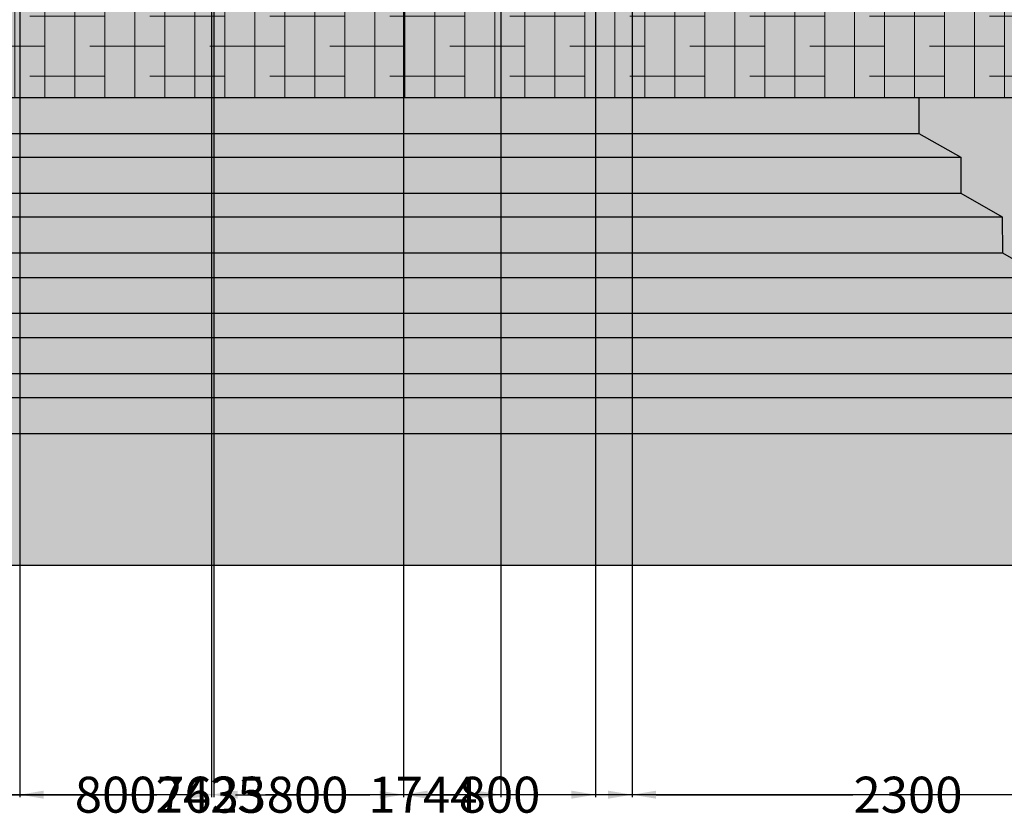
# Model space of a CAD drawing. Units: millimetres. Extents: x 11032 to 26788, y 3406 to 24505.
# Tile 12 of 78: x 17145 to 21249, y 3406 to 6736. Entities that reach past the tile are written whole.
import ezdxf

# ---------------------------------------------------------------- set-up
doc = ezdxf.new("R2010")
doc.units = ezdxf.units.MM
doc.header["$MEASUREMENT"] = 0
for name, color, linetype, lineweight in [('A-ANNO-DIMS', 2, 'Continuous', 18), ('A-FLOR-STRS', 7, 'Continuous', 25), ('A-FLOR-STRS-PATT', 8, 'Continuous', 13), ('A-WALL-PLIN', 7, 'Continuous', 30), ('A-WALL-PLIN-PATT', 253, 'Continuous', 13), ('L-PLNT-PATT', 92, 'Continuous', 13)]:
    doc.layers.add(name, color=color, linetype=linetype, lineweight=lineweight)
doc.styles.get("Standard").update_dxf_attribs({"font": 'arial.ttf'})
doc.dimstyles.get("Standard").update_dxf_attribs({"dimtxt": 150, "dimasz": 100, "dimexe": 10, "dimexo": 5, "dimgap": 5, "dimtad": 0, "dimtih": 1, "dimtoh": 1, "dimdec": 0, "dimzin": 0, "dimdsep": 46, "dimtxsty": 'Standard', "dimcen": 0.09, "dimadec": 0, "dimazin": 0, "dimtfac": 1, "dimtdec": 0, "dimtofl": 0, "dimtmove": 0, "dimatfit": 3, "dimfxl": 1, "dimtolj": 1, "dimtzin": 0, "dimarcsym": 0})

# ---------------------------------------------------------------- blocks, each defined once
blk = doc.blocks.new('*D36')
at = {"layer": 'A-ANNO-DIMS', "color": 0, "lineweight": -2, "transparency": 16777216}
for p, q in [((12301.3, 17115.9), (12301.3, 24416.9)), ((12401.3, 24406.9), (18569.2, 24406.9)), ((25297.4, 24406.9), (19129.5, 24406.9)), ((25397.4, 4466.4), (25397.4, 24416.9))]:
    blk.add_line(p, q, dxfattribs=at)
at = {"layer": 'A-ANNO-DIMS', "color": 0, "transparency": 16777216}
for points in [[(12401.3, 24423.5), (12401.3, 24390.2), (12301.3, 24406.9)], [(25297.4, 24423.5), (25297.4, 24390.2), (25397.4, 24406.9)]]:
    blk.add_solid(points, dxfattribs=at)
at = {"layer": 'Defpoints', "color": 0, "transparency": 16777216}
for p in [(25397.4, 24406.9), (12301.3, 17110.9), (25397.4, 4461.4)]:
    blk.add_point(p, dxfattribs=at)
at = {"layer": 'A-ANNO-DIMS', "color": 0, "transparency": 16777216, "insert": (18849.3, 24406.9), "char_height": 150, "attachment_point": 5}
blk.add_mtext('\\A1;13096', dxfattribs=at)
blk = doc.blocks.new('*D37')
at = {"layer": 'A-ANNO-DIMS', "color": 0, "lineweight": -2, "transparency": 16777216}
for p, q in [((18087.7, 23450.4), (11334.8, 23450.4)), ((11344.8, 23350.4), (11344.8, 14037.5)), ((11344.8, 4561.4), (11344.8, 13874.3)), ((12927.7, 4461.4), (11334.8, 4461.4))]:
    blk.add_line(p, q, dxfattribs=at)
at = {"layer": 'A-ANNO-DIMS', "color": 0, "transparency": 16777216}
for points in [[(11328.1, 23350.4), (11361.4, 23350.4), (11344.8, 23450.4)], [(11328.1, 4561.4), (11361.4, 4561.4), (11344.8, 4461.4)]]:
    blk.add_solid(points, dxfattribs=at)
at = {"layer": 'Defpoints', "color": 0, "transparency": 16777216}
for p in [(11344.8, 23450.4), (18092.7, 23450.4), (12932.7, 4461.4)]:
    blk.add_point(p, dxfattribs=at)
at = {"layer": 'A-ANNO-DIMS', "color": 0, "transparency": 16777216, "insert": (11344.8, 13955.9), "char_height": 150, "attachment_point": 5}
blk.add_mtext('\\A1;18989', dxfattribs=at)
blk = doc.blocks.new('*D49')
at = {"layer": 'A-ANNO-DIMS', "color": 0, "lineweight": -2, "transparency": 16777216}
for p, q in [((17953.5, 10206.4), (17953.5, 3494.9)), ((14996.4, 6406.4), (14996.4, 3494.9)), ((15096.4, 3504.9), (16244.7, 3504.9)), ((17853.5, 3504.9), (16705.2, 3504.9))]:
    blk.add_line(p, q, dxfattribs=at)
at = {"layer": 'A-ANNO-DIMS', "color": 0, "transparency": 16777216}
for points in [[(15096.4, 3521.6), (15096.4, 3488.2), (14996.4, 3504.9)], [(17853.5, 3521.6), (17853.5, 3488.2), (17953.5, 3504.9)]]:
    blk.add_solid(points, dxfattribs=at)
at = {"layer": 'Defpoints', "color": 0, "transparency": 16777216}
for p in [(17953.5, 10211.4), (14996.4, 6411.4), (17953.5, 3504.9)]:
    blk.add_point(p, dxfattribs=at)
at = {"layer": 'A-ANNO-DIMS', "color": 0, "transparency": 16777216, "insert": (16474.9, 3504.9), "char_height": 150, "attachment_point": 5}
blk.add_mtext('\\A1;2957', dxfattribs=at)
blk = doc.blocks.new('*D50')
at = {"layer": 'A-ANNO-DIMS', "color": 0, "lineweight": -2, "transparency": 16777216}
for p, q in [((19697.4, 16000.7), (19697.4, 3494.9)), ((17953.5, 10206.4), (17953.5, 3494.9)), ((18053.5, 3504.9), (18603.8, 3504.9)), ((19597.4, 3504.9), (19047, 3504.9))]:
    blk.add_line(p, q, dxfattribs=at)
at = {"layer": 'A-ANNO-DIMS', "color": 0, "transparency": 16777216}
for points in [[(18053.5, 3521.6), (18053.5, 3488.2), (17953.5, 3504.9)], [(19597.4, 3521.6), (19597.4, 3488.2), (19697.4, 3504.9)]]:
    blk.add_solid(points, dxfattribs=at)
at = {"layer": 'Defpoints', "color": 0, "transparency": 16777216}
for p in [(19697.4, 16005.7), (17953.5, 10211.4), (19697.4, 3504.9)]:
    blk.add_point(p, dxfattribs=at)
at = {"layer": 'A-ANNO-DIMS', "color": 0, "transparency": 16777216, "insert": (18825.4, 3504.9), "char_height": 150, "attachment_point": 5}
blk.add_mtext('\\A1;1744', dxfattribs=at)
blk = doc.blocks.new('*D51')
at = {"layer": 'A-ANNO-DIMS', "color": 0, "lineweight": -2, "transparency": 16777216}
for p, q in [((21997.4, 16011.6), (21997.4, 3494.9)), ((19697.4, 16000.7), (19697.4, 3494.9)), ((19797.4, 3504.9), (20617.4, 3504.9)), ((21897.4, 3504.9), (21077.4, 3504.9))]:
    blk.add_line(p, q, dxfattribs=at)
at = {"layer": 'A-ANNO-DIMS', "color": 0, "transparency": 16777216}
for points in [[(19797.4, 3521.6), (19797.4, 3488.2), (19697.4, 3504.9)], [(21897.4, 3521.6), (21897.4, 3488.2), (21997.4, 3504.9)]]:
    blk.add_solid(points, dxfattribs=at)
at = {"layer": 'Defpoints', "color": 0, "transparency": 16777216}
for p in [(21997.4, 16016.6), (19697.4, 16005.7), (21997.4, 3504.9)]:
    blk.add_point(p, dxfattribs=at)
at = {"layer": 'A-ANNO-DIMS', "color": 0, "transparency": 16777216, "insert": (20847.4, 3504.9), "char_height": 150, "attachment_point": 5}
blk.add_mtext('\\A1;2300', dxfattribs=at)
blk = doc.blocks.new('*D55')
at = {"layer": 'A-ANNO-DIMS', "color": 0, "lineweight": -2, "transparency": 16777216}
for p, q in [((14128.4, 5006.1), (14128.4, 3494.9)), ((21761, 5006.1), (21761, 3494.9)), ((14228.4, 3504.9), (17716.3, 3504.9)), ((21661, 3504.9), (18173.1, 3504.9))]:
    blk.add_line(p, q, dxfattribs=at)
at = {"layer": 'A-ANNO-DIMS', "color": 0, "transparency": 16777216}
for points in [[(14228.4, 3521.6), (14228.4, 3488.2), (14128.4, 3504.9)], [(21661, 3521.6), (21661, 3488.2), (21761, 3504.9)]]:
    blk.add_solid(points, dxfattribs=at)
at = {"layer": 'Defpoints', "color": 0, "transparency": 16777216}
for p in [(14128.4, 5011.1), (21761, 5011.1), (21761, 3504.9)]:
    blk.add_point(p, dxfattribs=at)
at = {"layer": 'A-ANNO-DIMS', "color": 0, "transparency": 16777216, "insert": (17944.7, 3504.9), "char_height": 150, "attachment_point": 5}
blk.add_mtext('\\A1;7633', dxfattribs=at)
blk = doc.blocks.new('*D58')
at = {"layer": 'A-ANNO-DIMS', "color": 0, "lineweight": -2, "transparency": 16777216}
for p, q in [((20899.7, 7261.4), (26363.9, 7261.4)), ((26353.9, 7161.4), (26353.9, 6918)), ((26353.9, 6511.4), (26353.9, 6754.8)), ((20898, 6411.4), (26363.9, 6411.4))]:
    blk.add_line(p, q, dxfattribs=at)
at = {"layer": 'A-ANNO-DIMS', "color": 0, "transparency": 16777216}
for points in [[(26337.2, 7161.4), (26370.6, 7161.4), (26353.9, 7261.4)], [(26337.2, 6511.4), (26370.6, 6511.4), (26353.9, 6411.4)]]:
    blk.add_solid(points, dxfattribs=at)
at = {"layer": 'Defpoints', "color": 0, "transparency": 16777216}
for p in [(20894.7, 7261.4), (26353.9, 7261.4), (20893, 6411.4)]:
    blk.add_point(p, dxfattribs=at)
at = {"layer": 'A-ANNO-DIMS', "color": 0, "transparency": 16777216, "insert": (26353.9, 6836.4), "char_height": 150, "attachment_point": 5}
blk.add_mtext('\\A1;850', dxfattribs=at)
blk = doc.blocks.new('*D62')
at = {"layer": 'A-ANNO-DIMS', "color": 0, "lineweight": -2, "transparency": 16777216}
for p, q in [((17144.7, 7306.4), (17144.7, 3494.9)), ((17944.7, 7256.4), (17944.7, 3494.9)), ((17244.7, 3504.9), (17374.2, 3504.9)), ((17844.7, 3504.9), (17715.3, 3504.9))]:
    blk.add_line(p, q, dxfattribs=at)
at = {"layer": 'A-ANNO-DIMS', "color": 0, "transparency": 16777216}
for points in [[(17244.7, 3521.6), (17244.7, 3488.2), (17144.7, 3504.9)], [(17844.7, 3521.6), (17844.7, 3488.2), (17944.7, 3504.9)]]:
    blk.add_solid(points, dxfattribs=at)
at = {"layer": 'Defpoints', "color": 0, "transparency": 16777216}
for p in [(17144.7, 7311.4), (17944.7, 7261.4), (17944.7, 3504.9)]:
    blk.add_point(p, dxfattribs=at)
at = {"layer": 'A-ANNO-DIMS', "color": 0, "transparency": 16777216, "insert": (17544.7, 3504.9), "char_height": 150, "attachment_point": 5}
blk.add_mtext('\\A1;800', dxfattribs=at)
blk = doc.blocks.new('*D63')
at = {"layer": 'A-ANNO-DIMS', "color": 0, "lineweight": -2, "transparency": 16777216}
for p, q in [((17944.7, 7256.4), (17944.7, 3494.9)), ((18744.7, 7256.4), (18744.7, 3494.9)), ((18044.7, 3504.9), (18174.2, 3504.9)), ((18644.7, 3504.9), (18515.3, 3504.9))]:
    blk.add_line(p, q, dxfattribs=at)
at = {"layer": 'A-ANNO-DIMS', "color": 0, "transparency": 16777216}
for points in [[(18044.7, 3521.6), (18044.7, 3488.2), (17944.7, 3504.9)], [(18644.7, 3521.6), (18644.7, 3488.2), (18744.7, 3504.9)]]:
    blk.add_solid(points, dxfattribs=at)
at = {"layer": 'Defpoints', "color": 0, "transparency": 16777216}
for p in [(17944.7, 7261.4), (18744.7, 7261.4), (18744.7, 3504.9)]:
    blk.add_point(p, dxfattribs=at)
at = {"layer": 'A-ANNO-DIMS', "color": 0, "transparency": 16777216, "insert": (18344.7, 3504.9), "char_height": 150, "attachment_point": 5}
blk.add_mtext('\\A1;800', dxfattribs=at)
blk = doc.blocks.new('*D64')
at = {"layer": 'A-ANNO-DIMS', "color": 0, "lineweight": -2, "transparency": 16777216}
for p, q in [((18744.7, 7256.4), (18744.7, 3494.9)), ((19544.7, 7256.4), (19544.7, 3494.9)), ((18844.7, 3504.9), (18974.2, 3504.9)), ((19444.7, 3504.9), (19315.3, 3504.9))]:
    blk.add_line(p, q, dxfattribs=at)
at = {"layer": 'A-ANNO-DIMS', "color": 0, "transparency": 16777216}
for points in [[(18844.7, 3521.6), (18844.7, 3488.2), (18744.7, 3504.9)], [(19444.7, 3521.6), (19444.7, 3488.2), (19544.7, 3504.9)]]:
    blk.add_solid(points, dxfattribs=at)
at = {"layer": 'Defpoints', "color": 0, "transparency": 16777216}
for p in [(18744.7, 7261.4), (19544.7, 7261.4), (19544.7, 3504.9)]:
    blk.add_point(p, dxfattribs=at)
at = {"layer": 'A-ANNO-DIMS', "color": 0, "transparency": 16777216, "insert": (19144.7, 3504.9), "char_height": 150, "attachment_point": 5}
blk.add_mtext('\\A1;800', dxfattribs=at)
blk = doc.blocks.new('*D66')
at = {"layer": 'A-ANNO-DIMS', "color": 0, "lineweight": -2, "transparency": 16777216}
for p, q in [((16725.9, 10296), (16725.9, 3494.9)), ((19150.9, 10296), (19150.9, 3494.9)), ((16825.9, 3504.9), (17707.6, 3504.9)), ((19050.9, 3504.9), (18169.3, 3504.9))]:
    blk.add_line(p, q, dxfattribs=at)
at = {"layer": 'A-ANNO-DIMS', "color": 0, "transparency": 16777216}
for points in [[(16825.9, 3521.6), (16825.9, 3488.2), (16725.9, 3504.9)], [(19050.9, 3521.6), (19050.9, 3488.2), (19150.9, 3504.9)]]:
    blk.add_solid(points, dxfattribs=at)
at = {"layer": 'Defpoints', "color": 0, "transparency": 16777216}
for p in [(16725.9, 10301), (19150.9, 10301), (19150.9, 3504.9)]:
    blk.add_point(p, dxfattribs=at)
at = {"layer": 'A-ANNO-DIMS', "color": 0, "transparency": 16777216, "insert": (17938.4, 3504.9), "char_height": 150, "attachment_point": 5}
blk.add_mtext('\\A1;2425', dxfattribs=at)

msp = doc.modelspace()

# ---------------------------------------------------------------- hatches: boundary and pattern name
at = {"layer": 'A-FLOR-STRS-PATT'}
h = msp.add_hatch(color=256, dxfattribs=at)
h.set_gradient(color1=(99, 100, 102), color2=(199, 200, 202), name='INVCYLINDER')
h.paths.add_polyline_path([(14996.399, 6411.399), (14996.399, 6261.399), (20893.008, 6261.399), (20893.008, 6411.399)])
h.paths.add_polyline_path([(21067.183, 6012.807), (21067.019, 6162.807), (14822.389, 6162.807), (14822.224, 6012.807)])
h.paths.add_polyline_path([(21241.977, 5763.336), (21240.69, 5913.331), (14648.718, 5913.331), (14647.43, 5763.336)])
h.paths.add_polyline_path([(14474.774, 5661.399), (14474.964, 5512.395), (21414.443, 5512.395), (21414.634, 5661.399)])
h.paths.add_polyline_path([(14302.433, 5411.236), (14301.435, 5261.24), (21587.972, 5261.24), (21586.974, 5411.236)])
h.paths.add_polyline_path([(14128.313, 5161.097), (14128.428, 5011.097), (21760.979, 5011.097), (21761.094, 5161.097)])
at = {"layer": 'A-WALL-PLIN-PATT'}
h = msp.add_hatch(color=256, dxfattribs=at)
h.set_gradient(color1=(99, 100, 102), color2=(199, 200, 202), name='CYLINDER')
edge = h.paths.add_edge_path()
edge.add_arc((17944.704, 7261.399), 2950, 180, 181.942602)
edge.add_line((14996.399, 7161.399), (12932.665, 7161.399))
edge.add_line((12932.665, 7161.399), (12932.665, 6411.399))
edge.add_line((12932.665, 6411.399), (25397.404, 6411.399))
edge.add_line((25397.404, 6411.399), (25397.404, 7161.399))
edge.add_line((25397.404, 7161.399), (22955.171, 7161.399))
edge.add_spline(control_points=[(22955.171, 7161.399), (22875.95, 7159.113), (22796.729, 7156.828), (22718.347, 7161.399)], knot_values=[0, 0, 0, 0, 236.62389499, 236.62389499, 236.62389499, 236.62389499], degree=3, periodic=0)
edge.add_spline(control_points=[(22718.347, 7161.399), (22709.27, 7161.929), (22517.84, 7175.049), (22332.009, 7233.921), (22155.123, 7291.176)], knot_values=[236.62389499, 236.62389499, 236.62389499, 236.62389499, 264.02785008, 815.24414583, 815.24414583, 815.24414583, 815.24414583], degree=3, periodic=0)
edge.add_line((22155.123, 7291.176), (22155.123, 7161.399))
edge.add_line((22155.123, 7161.399), (20893.008, 7161.399))
edge.add_arc((17944.704, 7261.399), 2950, 358.057398, 360)
edge.add_line((20894.704, 7261.399), (14994.704, 7261.399))
h.paths.add_polyline_path([(14996.399, 6261.399), (14822.389, 6162.807), (21067.019, 6162.807), (20893.008, 6261.399)])
h.paths.add_polyline_path([(14822.224, 6012.807), (14648.718, 5913.331), (21240.69, 5913.331), (21067.183, 6012.807)])
h.paths.add_polyline_path([(21414.634, 5661.399), (21414.635, 5662.395), (21241.977, 5763.336), (14647.43, 5763.336), (14474.772, 5662.395), (14474.774, 5661.399)])
h.paths.add_polyline_path([(14474.964, 5512.395), (14302.433, 5411.236), (21586.974, 5411.236), (21414.443, 5512.395)])
h.paths.add_polyline_path([(14301.435, 5261.24), (14128.313, 5161.097), (21761.094, 5161.097), (21587.972, 5261.24)])
h.paths.add_polyline_path([(22722.526, 4461.399), (21760.979, 5011.097), (14128.428, 5011.097), (13166.882, 4461.399)])
h = msp.add_hatch(dxfattribs=at)
h.set_pattern_fill('ANSI38', color=256, scale=1000, angle=45, style=0)
edge = h.paths.add_edge_path()
edge.add_line((25397.404, 6411.399), (25397.404, 7161.399))
edge.add_line((25397.404, 7161.399), (22955.171, 7161.399))
edge.add_spline(control_points=[(22955.171, 7161.399), (22875.95, 7159.113), (22796.729, 7156.828), (22718.347, 7161.399)], knot_values=[0, 0, 0, 0, 236.62389499, 236.62389499, 236.62389499, 236.62389499], degree=3, periodic=0)
edge.add_spline(control_points=[(22718.347, 7161.399), (22709.27, 7161.929), (22517.84, 7175.049), (22332.009, 7233.921), (22155.123, 7291.176)], knot_values=[236.62389499, 236.62389499, 236.62389499, 236.62389499, 264.02785008, 815.24414583, 815.24414583, 815.24414583, 815.24414583], degree=3, periodic=0)
edge.add_line((22155.123, 7291.176), (22155.123, 7161.399))
edge.add_line((22155.123, 7161.399), (20893.008, 7161.399))
edge.add_arc((17944.704, 7261.399), 2950, 358.057398, 360)
edge.add_line((20894.704, 7261.399), (14994.704, 7261.399))
edge.add_arc((17944.704, 7261.399), 2950, 180, 181.942602)
edge.add_line((14996.399, 7161.399), (12932.665, 7161.399))
edge.add_line((12932.665, 7161.399), (12932.665, 6411.399))
edge.add_line((12932.665, 6411.399), (25397.404, 6411.399))
at = {"layer": 'L-PLNT-PATT'}
h = msp.add_hatch(color=256, dxfattribs=at)
h.set_gradient(color1=(19, 155, 72), color2=(0, 127, 0), name='HEMISPHERICAL')
h.paths.add_polyline_path([(20893.008, 6411.399), (20893.008, 6261.399), (21067.019, 6162.807), (21067.183, 6012.807), (21240.69, 5913.331), (21241.977, 5763.336), (21416.338, 5661.399), (21414.634, 5661.399), (21414.443, 5512.395), (21586.974, 5411.236), (21587.972, 5261.24), (21761.094, 5161.097), (21760.979, 5011.097), (22722.526, 4461.399), (25397.404, 4461.399), (25397.404, 6411.399)])

# ---------------------------------------------------------------- linework, layer by layer
at = {"layer": 'A-FLOR-STRS'}
for p, q in [((20893.008, 6411.399), (20893.008, 6261.399)), ((14996.399, 6261.399), (20893.008, 6261.399)), ((20893.008, 6261.399), (21067.019, 6162.807)), ((14822.389, 6162.807), (21067.019, 6162.807)), ((21067.019, 6162.807), (21067.183, 6012.807)), ((14822.224, 6012.807), (21067.183, 6012.807)), ((21067.183, 6012.807), (21240.69, 5913.331)), ((14648.718, 5913.331), (21240.69, 5913.331)), ((21240.69, 5913.331), (21241.977, 5763.336)), ((14647.43, 5763.336), (21241.977, 5763.336)), ((21241.977, 5763.336), (21414.635, 5662.395)), ((14474.774, 5661.399), (21414.634, 5661.399)), ((14474.964, 5512.395), (21414.443, 5512.395)), ((14302.433, 5411.236), (21586.974, 5411.236)), ((14301.435, 5261.24), (21587.972, 5261.24)), ((14128.313, 5161.097), (21761.094, 5161.097)), ((14128.428, 5011.097), (21760.979, 5011.097))]:
    msp.add_line(p, q, dxfattribs=at)
at = {"layer": 'A-WALL-PLIN'}
for p, q in [((12932.665, 6411.399), (25397.404, 6411.399)), ((12932.665, 4461.399), (25397.404, 4461.399))]:
    msp.add_line(p, q, dxfattribs=at)

# ---------------------------------------------------------------- dimensions: what is measured, and where the dimension line sits
at = {"layer": 'A-ANNO-DIMS'}
for base, p1, p2, picture, middle in [((25397.404, 24406.858), (12301.265, 17110.885), (25397.404, 4461.399), '*D36', (18849.334, 24406.858)), ((21997.404, 3504.899), (19697.404, 16005.71), (21997.404, 16016.562), '*D51', (20847.404, 3504.899)), ((19697.404, 3504.899), (17953.455, 10211.41), (19697.404, 16005.71), '*D50', (18825.429, 3504.899)), ((19150.949, 3504.899), (16725.949, 10301.016), (19150.949, 10301.016), '*D66', (17938.449, 3504.899)), ((17953.455, 3504.899), (14996.399, 6411.399), (17953.455, 10211.41), '*D49', (16474.927, 3504.899)), ((17944.704, 3504.899), (17144.704, 7311.399), (17944.704, 7261.399), '*D62', (17544.704, 3504.899)), ((18744.704, 3504.899), (17944.704, 7261.399), (18744.704, 7261.399), '*D63', (18344.704, 3504.899)), ((19544.704, 3504.899), (18744.704, 7261.399), (19544.704, 7261.399), '*D64', (19144.704, 3504.899)), ((21760.979, 3504.899), (14128.428, 5011.097), (21760.979, 5011.097), '*D55', (17944.704, 3504.899))]:
    dim = msp.add_linear_dim(base=base, p1=p1, p2=p2, dimstyle='Standard', override={"dimdec": 0, "dimlfac": 1, "dimrnd": 0, "dimzin": 0, "dimdsep": 46, "dimlunit": 2}, dxfattribs=at)
    dim.commit()
    dim.dimension.update_dxf_attribs({"geometry": picture, "text_midpoint": middle})
for base, p1, p2, picture, middle in [((11344.765, 23450.358), (12932.665, 4461.399), (18092.739, 23450.358), '*D37', (11344.765, 13955.879)), ((26353.904, 7261.399), (20893.008, 6411.399), (20894.704, 7261.399), '*D58', (26353.904, 6836.399))]:
    dim = msp.add_linear_dim(base=base, p1=p1, p2=p2, angle=90, dimstyle='Standard', override={"dimdec": 0, "dimlfac": 1, "dimrnd": 0, "dimzin": 0, "dimdsep": 46, "dimlunit": 2}, dxfattribs=at)
    dim.commit()
    dim.dimension.update_dxf_attribs({"geometry": picture, "text_midpoint": middle})

doc.saveas('drawing.dxf')
